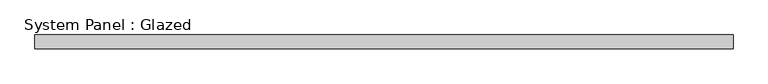
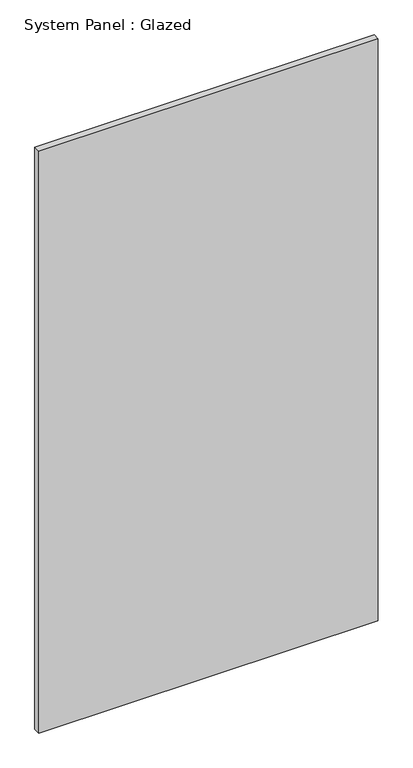
"""IFC4 building model written with IfcOpenShell, lengths in millimetres: plate geometry, System Panel : Glazed."""

from ifc_helpers import new_model, si_unit, origin, origin_with_axes, place, context, project, spatial, polyline, outline, extrude, source, transform, mapped, element, save


def system_panel_glazed_612c9cdf(model_context):
    return source(origin(), model_context, "Body", "SweptSolid", [
        extrude(outline(polyline([(638.175, 19.05), (-638.175, 19.05), (-638.175, 44.45), (638.175, 44.45), (638.175, 19.05)])), origin_with_axes(), (0.0, 0.0, 1.0), 2311.4),
    ])


if __name__ == "__main__":
    model = new_model("IFC4")
    model_context = context("Model", 3, world=origin())
    ifc_project = project(units=[si_unit("LENGTHUNIT", "METRE", prefix="MILLI")], contexts=[model_context])
    site = spatial("IfcSite", under=ifc_project)
    building = spatial("IfcBuilding", under=site)
    placement = place(None, origin())
    system_panel_glazed_shape = system_panel_glazed_612c9cdf(model_context)
    element("IfcPlate", 1, ObjectType="System Panel : Glazed", at=placement, inside=building, context=model_context, shape_type="MappedRepresentation", body=[
        mapped(system_panel_glazed_shape, transform((0.0, 0.0, 0.0), x_axis=(1.0, 0.0, 0.0), y_axis=(0.0, 1.0, 0.0), z_axis=(0.0, 0.0, 1.0))),
    ])
    save(model, "model.ifc")

# Revit data of these elements
# Type "System Panel : Glazed"
#   Construction Type Id = "GSP4R"
#   Analytic Construction = "1/8 in Pilkington single glazing"
#   Visual Light Transmittance = 0.9
#   Solar Heat Gain Coefficient = 0.86
#   Heat Transfer Coefficient (U) = 1.18115 BTU/(h·ft²·°F)
# Element 1 (IfcPlate, "System Panel : Glazed")
#   Materials on its faces: "Glass"
# Materials
#   "Glass": class "Glass", colour RGB 0 128 192, transparency 0.75, Description = "Soda Lime Glass", Cost = 0
